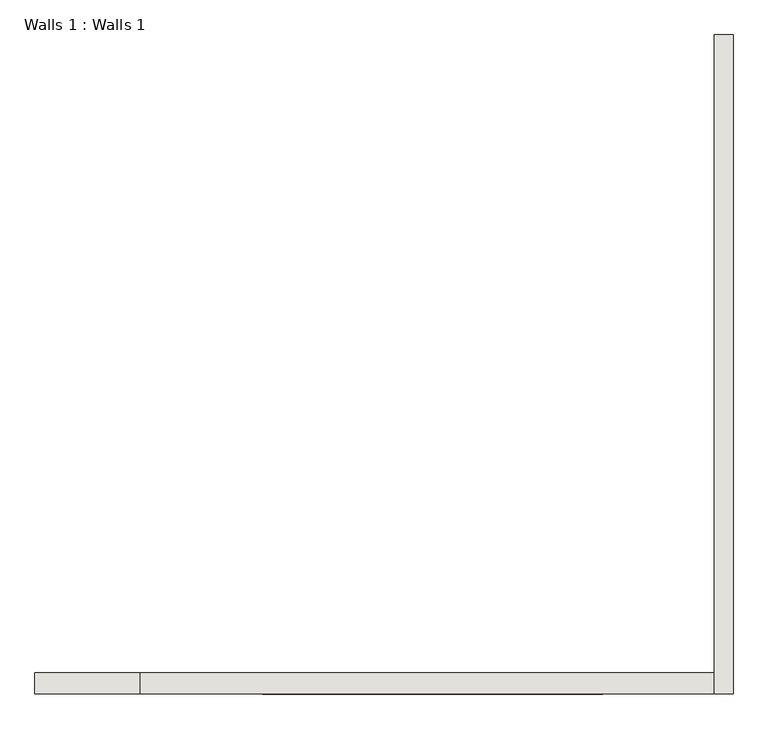
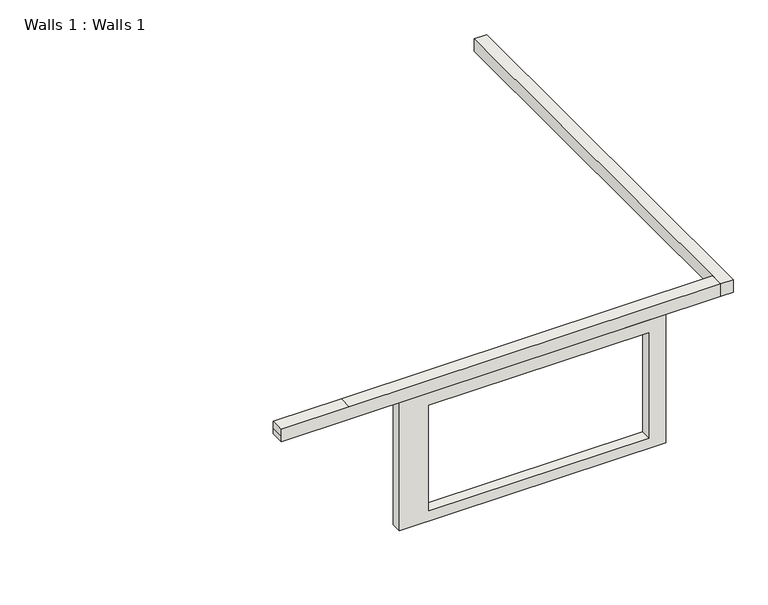
"""IFC4 building model written with IfcOpenShell, lengths in millimetres: wall geometry, Walls 1 : Walls 1."""

from ifc_helpers import new_model, si_unit, frame, origin, place, context, project, spatial, polyline, outline, extrude, source, transform, mapped, element, save


def walls_1_walls_1_3d42d239(model_context):
    return source(origin(), model_context, "Body", "SweptSolid", [
        extrude(outline(polyline([(2615.6828982, 7932.1740351), (2615.6828982, -4005.8259649), (2272.4271302, -4005.8259649), (2272.4271302, 7932.1740351), (2615.6828982, 7932.1740351)])), frame((0.0, 0.0, 7451.1408), z_axis=(0.0, 0.0, 1.0), x_axis=(1.0, 0.0, 0.0)), (0.0, 0.0, 1.0), 369.6113516),
        extrude(outline(polyline([(7820.7521516, 2272.4271302), (7820.7521516, -8116.1728698), (7820.7521516, -10021.335611), (7617.5521516, -10021.335611), (7451.1408, -10021.335611), (7451.1408, 2272.4271302), (7617.5521516, 2272.4271302), (7820.7521516, 2272.4271302)])), frame((0.0, -4005.8259649, 0.0), z_axis=(0.0, 1.0, 0.0), x_axis=(0.0, 0.0, 1.0)), (0.0, 0.0, 1.0), 381.0),
        extrude(outline(polyline([(7457.9778145, 273.867517), (7457.9778145, -6547.7228698), (7457.9778145, -6719.1728698), (3657.6, -6719.1728698), (3657.6, 734.1272116), (7457.9778145, 734.1272116), (7457.9778145, 273.867517)]), holes=[polyline([(7081.7433198, -5897.2145744), (7081.7433198, 258.2694807), (3962.4, 258.2694807), (3962.4, -5897.2145744), (7081.7433198, -5897.2145744)])]), frame((0.0, -4005.8259649, 0.0), z_axis=(0.0, 1.0, 0.0), x_axis=(0.0, 0.0, 1.0)), (0.0, 0.0, 1.0), 304.8),
    ])


if __name__ == "__main__":
    model = new_model("IFC4")
    model_context = context("Model", 3, world=origin())
    ifc_project = project(units=[si_unit("LENGTHUNIT", "METRE", prefix="MILLI")], contexts=[model_context])
    site = spatial("IfcSite", under=ifc_project)
    building = spatial("IfcBuilding", under=site)
    placement = place(None, origin())
    walls_1_walls_1_shape = walls_1_walls_1_3d42d239(model_context)
    element("IfcWall", 1, ObjectType="Walls 1 : Walls 1", at=placement, inside=building, context=model_context, shape_type="MappedRepresentation", body=[
        mapped(walls_1_walls_1_shape, transform((0.0, 0.0, 0.0), x_axis=(1.0, 0.0, 0.0), y_axis=(0.0, 1.0, 0.0), z_axis=(0.0, 0.0, 1.0))),
    ])
    save(model, "model.ifc")

# Revit data of these elements
# Element 1 (IfcWall, "Walls 1 : Walls 1")
#   Materials on its faces: "Default Wall"
# Materials
#   "Default Wall": colour RGB 128 128 128, transparency 0
